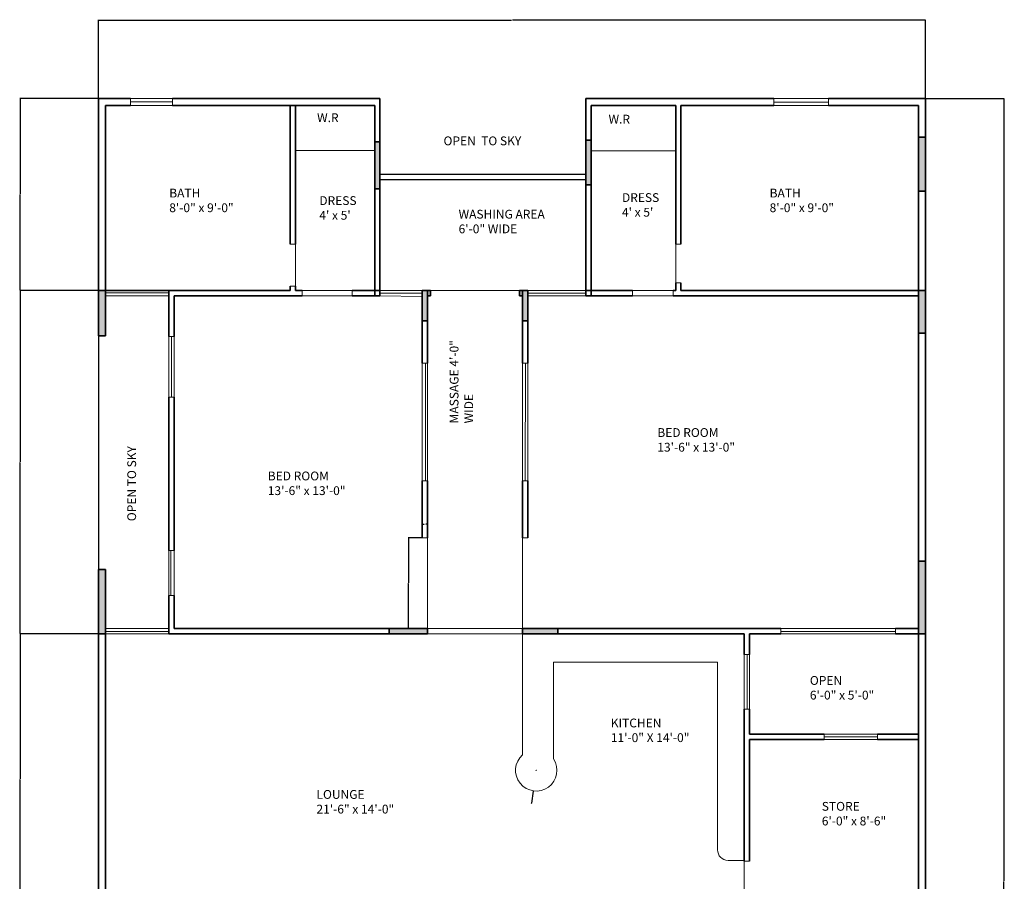
# Model space of a CAD drawing. Units: inches. Extents: x 1002 to 1561, y 1016 to 1994.
# Tile 8 of 8: x 1002 to 1561, y 1505 to 1994. Entities that reach past the tile are written whole.
import ezdxf

# ---------------------------------------------------------------- set-up
doc = ezdxf.new("R2010")
doc.units = ezdxf.units.IN
doc.header["$MEASUREMENT"] = 0
for name, color, linetype, lineweight in [('A-ANNO-DIMS', 2, 'Continuous', 18), ('A-AREA-IDEN', 7, 'Continuous', 18), ('A-WALL', 7, 'Continuous', 35), ('A-WALL-PATT', 7, 'Continuous', 13)]:
    doc.layers.add(name, color=color, linetype=linetype, lineweight=lineweight)
for name, color, linetype, lineweight, true_color in [('A-DOOR', 30, 'Continuous', 18, 0xf8991e), ('A-FLOR-CASE', 217, 'Continuous', 20, 0x93278f), ('A-FLOR-EDGE', 217, 'Continuous', 25, 0x93278f), ('A-GLAZ', 217, 'Continuous', 18, 0x93278f)]:
    doc.layers.add(name, color=color, linetype=linetype, lineweight=lineweight, true_color=true_color)
doc.styles.get("Standard").update_dxf_attribs({"font": 'arial.ttf'})
doc.dimstyles.get("Standard").update_dxf_attribs({"dimtxt": 0.18, "dimasz": 0.18, "dimexe": 0.18, "dimexo": 0.0625, "dimgap": 0.09, "dimtad": 0, "dimtih": 1, "dimtoh": 1, "dimdec": 4, "dimzin": 0, "dimdsep": 46, "dimtxsty": 'Standard', "dimcen": 0.09, "dimadec": 0, "dimazin": 0, "dimtfac": 1, "dimtdec": 4, "dimtofl": 0, "dimtmove": 0, "dimatfit": 3, "dimfxl": 1, "dimtolj": 1, "dimtzin": 0, "dimarcsym": 0})

# ---------------------------------------------------------------- blocks, each defined once
blk = doc.blocks.new('DOOR-PASSAGE-BEDROOM')
for p, q in [((0, 51.46), (3, 51.46)), ((3, 51.46), (3, 0))]:
    blk.add_line(p, q)
blk = doc.blocks.new('*D5')
at = {"layer": 'A-ANNO-DIMS', "color": 0, "lineweight": -2, "transparency": 16777216}
for p, q in [((1230.37, 1699.97), (1222.53, 1699.97)), ((1222.71, 1699.79), (1222.71, 1674.42)), ((1222.71, 1648.69), (1222.71, 1674.06)), ((1230.37, 1648.51), (1222.53, 1648.51))]:
    blk.add_line(p, q, dxfattribs=at)
at = {"layer": 'A-ANNO-DIMS', "color": 0, "transparency": 16777216}
for points in [[(1222.68, 1699.79), (1222.74, 1699.79), (1222.71, 1699.97)], [(1222.68, 1648.69), (1222.74, 1648.69), (1222.71, 1648.51)]]:
    blk.add_solid(points, dxfattribs=at)
at = {"layer": 'Defpoints', "color": 0, "transparency": 16777216}
for p in [(1222.71, 1699.97), (1230.43, 1699.97), (1230.43, 1648.51)]:
    blk.add_point(p, dxfattribs=at)
at = {"layer": 'A-ANNO-DIMS', "color": 0, "transparency": 16777216, "insert": (1222.71, 1674.24), "char_height": 0.18, "attachment_point": 5}
blk.add_mtext('\\A1;PASSAGE 51 TYP.', dxfattribs=at)
blk = doc.blocks.new('*D6')
at = {"layer": 'A-ANNO-DIMS', "color": 0, "lineweight": -2, "transparency": 16777216}
for p, q in [((1230.43, 1700.03), (1230.43, 1707.87)), ((1230.61, 1707.69), (1231.48, 1707.69)), ((1233.25, 1707.69), (1232.39, 1707.69)), ((1233.43, 1700.03), (1233.43, 1707.87))]:
    blk.add_line(p, q, dxfattribs=at)
at = {"layer": 'A-ANNO-DIMS', "color": 0, "transparency": 16777216}
for points in [[(1230.61, 1707.72), (1230.61, 1707.66), (1230.43, 1707.69)], [(1233.25, 1707.72), (1233.25, 1707.66), (1233.43, 1707.69)]]:
    blk.add_solid(points, dxfattribs=at)
at = {"layer": 'Defpoints', "color": 0, "transparency": 16777216}
for p in [(1233.43, 1707.69), (1230.43, 1699.97), (1233.43, 1699.97)]:
    blk.add_point(p, dxfattribs=at)
at = {"layer": 'A-ANNO-DIMS', "color": 0, "transparency": 16777216, "insert": (1231.93, 1707.69), "char_height": 0.18, "attachment_point": 5}
blk.add_mtext('\\A1;3 TYP.', dxfattribs=at)
blk = doc.blocks.new('*D7')
at = {"layer": 'A-ANNO-DIMS', "color": 0, "lineweight": -2, "transparency": 16777216}
for p, q in [((1046.43, 1949.57), (1046.43, 1994.2)), ((1046.61, 1994.02), (1281.14, 1994.02)), ((1516.25, 1994.02), (1281.73, 1994.02)), ((1516.43, 1949.57), (1516.43, 1994.2))]:
    blk.add_line(p, q, dxfattribs=at)
at = {"layer": 'A-ANNO-DIMS', "color": 0, "transparency": 16777216}
for points in [[(1046.61, 1994.05), (1046.61, 1993.99), (1046.43, 1994.02)], [(1516.25, 1994.05), (1516.25, 1993.99), (1516.43, 1994.02)]]:
    blk.add_solid(points, dxfattribs=at)
at = {"layer": 'Defpoints', "color": 0, "transparency": 16777216}
for p in [(1516.43, 1994.02), (1046.43, 1949.51), (1516.43, 1949.51)]:
    blk.add_point(p, dxfattribs=at)
at = {"layer": 'A-ANNO-DIMS', "color": 0, "transparency": 16777216, "insert": (1281.43, 1994.02), "char_height": 0.18, "attachment_point": 5}
blk.add_mtext('\\A1;470', dxfattribs=at)
blk = doc.blocks.new('*D8')
at = {"layer": 'A-ANNO-DIMS', "color": 0, "lineweight": -2, "transparency": 16777216}
for p, q in [((1516.5, 1949.51), (1561.12, 1949.51)), ((1560.94, 1949.33), (1560.94, 1505.18)), ((1560.94, 1060.67), (1560.94, 1504.82)), ((1472.5, 1060.49), (1561.12, 1060.49))]:
    blk.add_line(p, q, dxfattribs=at)
at = {"layer": 'A-ANNO-DIMS', "color": 0, "transparency": 16777216}
for points in [[(1560.91, 1949.33), (1560.97, 1949.33), (1560.94, 1949.51)], [(1560.91, 1060.67), (1560.97, 1060.67), (1560.94, 1060.49)]]:
    blk.add_solid(points, dxfattribs=at)
at = {"layer": 'Defpoints', "color": 0, "transparency": 16777216}
for p in [(1516.43, 1949.51), (1560.94, 1949.51), (1472.43, 1060.49)]:
    blk.add_point(p, dxfattribs=at)
at = {"layer": 'A-ANNO-DIMS', "color": 0, "transparency": 16777216, "insert": (1560.94, 1505), "char_height": 0.18, "attachment_point": 5}
blk.add_mtext('\\A1;889', dxfattribs=at)
blk = doc.blocks.new('*D9')
at = {"layer": 'A-ANNO-DIMS', "color": 0, "lineweight": -2, "transparency": 16777216}
for p, q in [((1046.37, 1949.51), (1001.74, 1949.51)), ((1001.92, 1949.33), (1001.92, 1895.19)), ((1001.92, 1840.69), (1001.92, 1894.83)), ((1046.37, 1840.51), (1001.74, 1840.51))]:
    blk.add_line(p, q, dxfattribs=at)
at = {"layer": 'A-ANNO-DIMS', "color": 0, "transparency": 16777216}
for points in [[(1001.89, 1949.33), (1001.95, 1949.33), (1001.92, 1949.51)], [(1001.89, 1840.69), (1001.95, 1840.69), (1001.92, 1840.51)]]:
    blk.add_solid(points, dxfattribs=at)
at = {"layer": 'Defpoints', "color": 0, "transparency": 16777216}
for p in [(1001.92, 1949.51), (1046.43, 1949.51), (1046.43, 1840.51)]:
    blk.add_point(p, dxfattribs=at)
at = {"layer": 'A-ANNO-DIMS', "color": 0, "transparency": 16777216, "insert": (1001.92, 1895.01), "char_height": 0.18, "attachment_point": 5}
blk.add_mtext('\\A1;109', dxfattribs=at)
blk = doc.blocks.new('*D10')
at = {"layer": 'A-ANNO-DIMS', "color": 0, "lineweight": -2, "transparency": 16777216}
for p, q in [((1046.37, 1840.51), (1001.74, 1840.51)), ((1001.92, 1840.33), (1001.92, 1743.19)), ((1001.92, 1645.69), (1001.92, 1742.83)), ((1046.37, 1645.51), (1001.74, 1645.51))]:
    blk.add_line(p, q, dxfattribs=at)
at = {"layer": 'A-ANNO-DIMS', "color": 0, "transparency": 16777216}
for points in [[(1001.89, 1840.33), (1001.95, 1840.33), (1001.92, 1840.51)], [(1001.89, 1645.69), (1001.95, 1645.69), (1001.92, 1645.51)]]:
    blk.add_solid(points, dxfattribs=at)
at = {"layer": 'Defpoints', "color": 0, "transparency": 16777216}
for p in [(1001.92, 1840.51), (1046.43, 1840.51), (1046.43, 1645.51)]:
    blk.add_point(p, dxfattribs=at)
at = {"layer": 'A-ANNO-DIMS', "color": 0, "transparency": 16777216, "insert": (1001.92, 1743.01), "char_height": 0.18, "attachment_point": 5}
blk.add_mtext('\\A1;195', dxfattribs=at)
blk = doc.blocks.new('*D11')
at = {"layer": 'A-ANNO-DIMS', "color": 0, "lineweight": -2, "transparency": 16777216}
for p, q in [((1046.37, 1645.51), (1001.74, 1645.51)), ((1001.92, 1645.33), (1001.92, 1563.19)), ((1001.92, 1480.69), (1001.92, 1562.83)), ((1046.37, 1480.51), (1001.74, 1480.51))]:
    blk.add_line(p, q, dxfattribs=at)
at = {"layer": 'A-ANNO-DIMS', "color": 0, "transparency": 16777216}
for points in [[(1001.89, 1645.33), (1001.95, 1645.33), (1001.92, 1645.51)], [(1001.89, 1480.69), (1001.95, 1480.69), (1001.92, 1480.51)]]:
    blk.add_solid(points, dxfattribs=at)
at = {"layer": 'Defpoints', "color": 0, "transparency": 16777216}
for p in [(1001.92, 1645.51), (1046.43, 1645.51), (1046.43, 1480.51)]:
    blk.add_point(p, dxfattribs=at)
at = {"layer": 'A-ANNO-DIMS', "color": 0, "transparency": 16777216, "insert": (1001.92, 1563.01), "char_height": 0.18, "attachment_point": 5}
blk.add_mtext('\\A1;165', dxfattribs=at)
blk = doc.blocks.new('*D22')
at = {"layer": 'A-ANNO-DIMS', "color": 0, "lineweight": -2, "transparency": 16777216}
for p, q in [((1295.12, 1568.03), (1295.3, 1568.03)), ((1295.21, 1567.94), (1295.21, 1568.12)), ((1292.67, 1549.35), (1293.6, 1556.18)), ((1292.49, 1549.35), (1292.67, 1549.35))]:
    blk.add_line(p, q, dxfattribs=at)
at = {"layer": 'A-ANNO-DIMS', "color": 0, "transparency": 16777216}
blk.add_solid([(1293.57, 1556.18), (1293.63, 1556.17), (1293.63, 1556.35)], dxfattribs=at)
at = {"layer": 'Defpoints', "color": 0, "transparency": 16777216}
for p in [(1295.21, 1568.03), (1293.63, 1556.35)]:
    blk.add_point(p, dxfattribs=at)
at = {"layer": 'A-ANNO-DIMS', "color": 0, "transparency": 16777216, "insert": (1292.01, 1549.35), "char_height": 0.18, "attachment_point": 5}
blk.add_mtext('\\A1;R11.78', dxfattribs=at)

msp = doc.modelspace()

# ---------------------------------------------------------------- hatches: boundary and pattern name
at = {"layer": 'A-WALL-PATT'}
h = msp.add_hatch(color=256, dxfattribs=at)
h.dxf.hatch_style = 1
h.paths.add_polyline_path([(1206.434, 1924.784), (1203.434, 1924.784), (1203.434, 1898.155), (1206.434, 1898.155)])
h.paths.add_polyline_path([(1326.434, 1925.745), (1323.434, 1925.745), (1323.434, 1900.458), (1326.434, 1900.458)])
h.paths.add_polyline_path([(1290.434, 1840.51), (1287.434, 1840.51), (1287.434, 1837.51), (1287.434, 1823.284), (1290.434, 1823.284)])
h.paths.add_polyline_path([(1287.434, 1840.51), (1285.684, 1840.51), (1285.684, 1837.51), (1287.434, 1837.51)])
h.paths.add_polyline_path([(1233.434, 1840.51), (1230.434, 1840.51), (1230.434, 1823.284), (1233.434, 1823.284)])
h.paths.add_polyline_path([(1235.119, 1840.51), (1233.434, 1840.51), (1233.434, 1837.51), (1235.119, 1837.51)])
h.paths.add_polyline_path([(1050.434, 1837.51), (1050.434, 1840.51), (1046.434, 1840.51), (1046.434, 1814.619), (1050.434, 1814.619)])
h.paths.add_polyline_path([(1050.434, 1682.088), (1046.434, 1682.088), (1046.434, 1648.51), (1046.434, 1645.51), (1050.434, 1645.51), (1050.434, 1648.51)])
h.paths.add_polyline_path([(1233.434, 1648.51), (1211.636, 1648.51), (1211.636, 1645.51), (1233.434, 1645.51)])
h.paths.add_polyline_path([(1307.549, 1648.51), (1287.434, 1648.51), (1287.434, 1645.51), (1307.549, 1645.51)])
h.paths.add_polyline_path([(1516.434, 1927.595), (1512.434, 1927.595), (1512.434, 1896.846), (1516.434, 1896.846)])
h.paths.add_polyline_path([(1516.434, 1840.51), (1512.434, 1840.51), (1512.434, 1816.31), (1516.434, 1816.31)])
h.paths.add_polyline_path([(1516.434, 1686.827), (1512.434, 1686.827), (1512.434, 1645.51), (1516.434, 1645.51)])
h.paths.add_polyline_path([(1472.434, 1321.51), (1469.434, 1321.51), (1469.434, 1306.51), (1472.434, 1306.51)])
h.paths.add_polyline_path([(1295.733, 1141.51), (1281.793, 1141.51), (1281.793, 1137.51), (1295.733, 1137.51)])
h.paths.add_polyline_path([(1239.434, 1321.51), (1230.434, 1321.51), (1230.434, 1318.51), (1239.434, 1318.51)])
h.paths.add_polyline_path([(1290.434, 1332.122), (1287.434, 1332.122), (1287.434, 1318.51), (1290.434, 1318.51)])
h.paths.add_polyline_path([(1311.434, 1480.51), (1287.434, 1480.51), (1287.434, 1477.51), (1311.434, 1477.51)])
h.paths.add_polyline_path([(1050.434, 1480.51), (1046.434, 1480.51), (1046.434, 1468.51), (1050.434, 1468.51)])
h.paths.add_polyline_path([(1050.434, 1321.51), (1046.434, 1321.51), (1046.434, 1309.51), (1050.434, 1309.51)])
h.paths.add_polyline_path([(1233.434, 1192.382), (1230.434, 1192.382), (1230.434, 1168.702), (1233.434, 1168.702)])
h.paths.add_polyline_path([(1050.434, 1137.51), (1046.434, 1137.51), (1046.434, 1119.51), (1050.434, 1119.51)])
h.paths.add_polyline_path([(1472.434, 1153.51), (1469.434, 1153.51), (1469.434, 1141.51), (1472.434, 1141.51)])
h.paths.add_polyline_path([(1472.434, 1141.51), (1469.434, 1141.51), (1469.434, 1137.51), (1472.434, 1137.51)])

# ---------------------------------------------------------------- linework, layer by layer
at = {"layer": 'A-DOOR'}
for p, q in [((1155.434, 1866.825), (1158.434, 1866.825)), ((1158.434, 1866.825), (1158.434, 1842.825)), ((1374.434, 1866.761), (1377.434, 1866.761)), ((1374.434, 1866.761), (1374.434, 1844.738)), ((1377.434, 1866.761), (1377.434, 1866.761)), ((1155.434, 1842.825), (1158.434, 1842.825)), ((1158.434, 1842.825), (1158.434, 1844.508)), ((1374.434, 1844.738), (1377.434, 1844.738)), ((1162.17, 1840.51), (1162.17, 1837.51)), ((1162.17, 1837.51), (1162.17, 1840.51)), ((1162.17, 1840.51), (1190.563, 1840.51)), ((1162.17, 1837.51), (1162.17, 1838.97)), ((1162.17, 1837.51), (1162.17, 1837.51)), ((1190.563, 1837.51), (1162.17, 1837.51)), ((1190.563, 1840.51), (1190.563, 1837.51)), ((1190.563, 1840.51), (1190.563, 1840.51)), ((1190.563, 1840.51), (1190.563, 1837.51)), ((1230.434, 1840.51), (1290.434, 1840.51)), ((1349.824, 1840.51), (1349.824, 1837.51)), ((1349.824, 1840.51), (1373.044, 1840.51)), ((1349.824, 1837.51), (1349.824, 1840.51)), ((1373.044, 1837.51), (1349.824, 1837.51)), ((1373.044, 1840.51), (1373.044, 1837.51)), ((1373.044, 1840.51), (1373.044, 1837.51)), ((1233.434, 1648.51), (1287.434, 1648.51)), ((1233.434, 1648.51), (1233.434, 1648.51)), ((1233.434, 1645.51), (1287.434, 1645.51)), ((1413.434, 1482.91), (1413.434, 1516.898)), ((1413.434, 1516.51), (1416.434, 1516.51))]:
    msp.add_line(p, q, dxfattribs=at)
at = {"layer": 'A-FLOR-CASE'}
for p, q in [((1158.434, 1919.94), (1203.434, 1919.94)), ((1326.434, 1919.822), (1374.434, 1919.822)), ((1287.434, 1645.51), (1287.434, 1576.873)), ((1305.105, 1574.472), (1305.105, 1629.469)), ((1305.105, 1629.469), (1398.202, 1629.469)), ((1398.202, 1629.469), (1398.202, 1522.898)), ((1305.075, 1574.472), (1305.105, 1574.472)), ((1404.202, 1516.898), (1413.434, 1516.898))]:
    msp.add_line(p, q, dxfattribs=at)
for centre, radius, start, end in [((1295.214, 1568.028), 11.78, 131.33697, 33.16787), ((1404.202, 1522.898), 6, 180, 270)]:
    msp.add_arc(centre, radius, start, end, dxfattribs=at)
at = {"layer": 'A-FLOR-EDGE'}
for p, q in [((1206.434, 1906.51), (1323.434, 1906.51)), ((1206.434, 1903.51), (1323.434, 1903.51)), ((1046.434, 1814.619), (1046.434, 1682.088))]:
    msp.add_line(p, q, dxfattribs=at)
at = {"layer": 'A-GLAZ'}
for p, q in [((1064.589, 1949.51), (1064.589, 1945.51)), ((1064.589, 1949.51), (1064.589, 1947.605)), ((1064.589, 1949.51), (1088.589, 1949.51)), ((1064.589, 1947.605), (1064.589, 1949.51)), ((1064.589, 1945.51), (1064.589, 1947.605)), ((1064.589, 1947.605), (1088.589, 1947.605)), ((1088.589, 1947.605), (1064.589, 1947.605)), ((1088.589, 1949.51), (1088.589, 1945.51)), ((1088.589, 1949.51), (1088.589, 1945.51)), ((1088.589, 1947.605), (1088.589, 1947.605)), ((1430.22, 1949.51), (1430.22, 1945.51)), ((1430.22, 1949.51), (1461.269, 1949.51)), ((1430.22, 1945.51), (1430.22, 1947.309)), ((1430.22, 1947.309), (1461.269, 1947.309)), ((1430.22, 1947.309), (1430.22, 1945.51)), ((1461.269, 1945.51), (1461.269, 1949.51)), ((1461.269, 1949.51), (1461.269, 1945.51)), ((1461.269, 1949.51), (1461.269, 1947.309)), ((1461.269, 1947.309), (1461.269, 1946.212)), ((1088.589, 1945.51), (1064.589, 1945.51)), ((1461.269, 1945.51), (1430.22, 1945.51)), ((1461.269, 1946.212), (1461.269, 1945.51)), ((1050.434, 1840.51), (1086.434, 1840.51)), ((1050.434, 1837.51), (1050.434, 1840.51)), ((1050.434, 1840.51), (1050.434, 1839.081)), ((1050.434, 1839.081), (1086.434, 1839.081)), ((1050.434, 1839.081), (1086.434, 1839.081)), ((1050.434, 1837.51), (1086.434, 1837.51)), ((1086.434, 1837.51), (1050.434, 1837.51)), ((1086.434, 1840.51), (1086.434, 1837.51)), ((1086.434, 1837.51), (1086.434, 1840.51)), ((1206.434, 1840.51), (1230.434, 1840.51)), ((1206.434, 1837.51), (1206.434, 1838.841)), ((1206.434, 1838.841), (1230.434, 1838.841)), ((1206.434, 1838.841), (1206.434, 1837.51)), ((1230.434, 1837.06), (1206.434, 1837.51)), ((1230.434, 1840.51), (1230.434, 1837.06)), ((1230.434, 1840.51), (1230.434, 1837.06)), ((1290.434, 1840.51), (1323.434, 1840.51)), ((1290.434, 1837.51), (1290.434, 1838.931)), ((1290.434, 1838.931), (1323.434, 1838.931)), ((1290.434, 1838.931), (1290.434, 1837.51)), ((1323.434, 1837.51), (1290.434, 1837.51)), ((1323.434, 1840.51), (1323.434, 1837.51)), ((1086.434, 1814.37), (1089.434, 1814.37)), ((1086.434, 1814.37), (1086.434, 1779.843)), ((1089.434, 1814.37), (1087.973, 1814.37)), ((1087.973, 1814.37), (1087.973, 1779.843)), ((1089.434, 1779.843), (1089.434, 1814.37)), ((1230.434, 1799.12), (1233.434, 1799.12)), ((1230.434, 1799.12), (1230.434, 1732.434)), ((1233.434, 1799.12), (1232.301, 1799.12)), ((1233.434, 1799.12), (1232.301, 1799.12)), ((1232.301, 1799.12), (1232.301, 1732.434)), ((1233.434, 1799.12), (1232.301, 1799.12)), ((1233.434, 1732.434), (1233.434, 1799.12)), ((1287.434, 1799.12), (1290.434, 1799.12)), ((1287.434, 1799.12), (1290.434, 1799.12)), ((1287.434, 1732.434), (1287.434, 1799.12)), ((1287.434, 1799.12), (1290.434, 1799.12)), ((1288.984, 1732.434), (1289.17, 1799.12)), ((1290.434, 1799.12), (1289.17, 1799.12)), ((1290.434, 1799.12), (1290.434, 1732.434)), ((1086.434, 1779.843), (1089.434, 1779.843)), ((1086.434, 1779.843), (1089.434, 1779.843)), ((1230.434, 1732.434), (1233.434, 1732.434)), ((1230.434, 1732.434), (1233.434, 1732.434)), ((1230.434, 1732.434), (1233.434, 1732.434)), ((1287.434, 1732.434), (1290.434, 1732.434)), ((1290.434, 1732.434), (1287.434, 1732.434)), ((1287.434, 1732.434), (1288.984, 1732.434)), ((1288.984, 1732.434), (1287.434, 1732.434)), ((1287.434, 1732.434), (1288.984, 1732.434)), ((1287.434, 1732.434), (1288.984, 1732.434)), ((1288.984, 1732.434), (1287.434, 1732.434)), ((1287.434, 1732.434), (1288.984, 1732.434)), ((1288.984, 1732.434), (1287.434, 1732.434)), ((1287.434, 1732.434), (1287.434, 1732.434)), ((1287.434, 1732.434), (1290.434, 1732.434)), ((1290.434, 1732.434), (1288.984, 1732.434)), ((1089.434, 1692.845), (1086.434, 1692.845)), ((1086.434, 1692.845), (1086.434, 1667.256)), ((1089.434, 1692.845), (1087.651, 1692.845)), ((1087.651, 1692.845), (1087.651, 1667.256)), ((1089.434, 1667.256), (1089.434, 1692.845)), ((1086.434, 1667.256), (1089.434, 1667.256)), ((1086.434, 1667.256), (1089.434, 1667.256)), ((1050.434, 1648.51), (1050.434, 1648.51)), ((1086.434, 1648.51), (1050.434, 1648.51)), ((1050.434, 1648.51), (1050.434, 1645.51)), ((1050.434, 1645.51), (1050.434, 1646.847)), ((1050.434, 1646.847), (1086.434, 1646.847)), ((1050.434, 1645.51), (1086.434, 1645.51)), ((1086.434, 1645.51), (1086.434, 1648.51)), ((1086.434, 1648.51), (1086.434, 1645.51)), ((1086.434, 1648.51), (1086.434, 1645.51)), ((1086.434, 1648.51), (1086.434, 1645.51)), ((1434.192, 1648.51), (1434.192, 1645.51)), ((1434.192, 1648.51), (1499.306, 1648.51)), ((1434.192, 1645.51), (1434.192, 1646.91)), ((1434.192, 1646.91), (1499.306, 1646.91)), ((1499.306, 1645.51), (1434.192, 1645.51)), ((1499.306, 1648.51), (1499.306, 1645.51)), ((1499.306, 1648.51), (1499.306, 1645.51)), ((1413.434, 1633.854), (1416.434, 1633.854)), ((1413.434, 1633.854), (1413.434, 1602.679)), ((1416.434, 1633.854), (1415.045, 1633.854)), ((1415.045, 1633.854), (1415.045, 1602.679)), ((1416.434, 1602.679), (1416.434, 1633.854)), ((1416.434, 1602.679), (1413.434, 1602.679)), ((1413.434, 1602.679), (1416.434, 1602.679)), ((1458.847, 1588.51), (1458.847, 1585.51)), ((1458.847, 1588.51), (1489.017, 1588.51)), ((1458.847, 1586.362), (1458.847, 1587.066)), ((1458.847, 1587.066), (1489.017, 1587.066)), ((1458.847, 1585.51), (1458.847, 1586.362)), ((1489.017, 1585.51), (1458.847, 1585.51)), ((1489.017, 1585.51), (1489.017, 1588.51)), ((1489.017, 1588.51), (1489.017, 1585.51))]:
    msp.add_line(p, q, dxfattribs=at)
at = {"layer": 'A-WALL'}
for p, q in [((1046.434, 1949.51), (1064.589, 1949.51)), ((1046.434, 1949.51), (1064.589, 1949.51)), ((1046.434, 1949.51), (1046.434, 1814.619)), ((1046.434, 1814.619), (1046.434, 1949.51)), ((1088.589, 1949.51), (1206.434, 1949.51)), ((1206.434, 1837.51), (1206.434, 1949.51)), ((1323.434, 1837.51), (1323.434, 1949.51)), ((1323.434, 1949.51), (1430.22, 1949.51)), ((1323.434, 1949.51), (1323.434, 1925.745)), ((1516.434, 1949.51), (1461.269, 1949.51)), ((1461.269, 1949.51), (1516.434, 1949.51)), ((1516.434, 1949.51), (1516.434, 1927.595)), ((1050.434, 1945.51), (1064.589, 1945.51)), ((1050.434, 1945.51), (1050.434, 1839.081)), ((1088.589, 1945.51), (1203.434, 1945.51)), ((1155.434, 1866.825), (1155.434, 1945.51)), ((1158.434, 1945.51), (1158.434, 1927.313)), ((1158.434, 1945.51), (1158.434, 1909.558)), ((1158.434, 1866.825), (1158.434, 1945.51)), ((1203.434, 1837.51), (1203.434, 1945.51)), ((1203.434, 1945.51), (1203.434, 1898.155)), ((1326.434, 1837.51), (1326.434, 1945.51)), ((1326.434, 1945.51), (1374.434, 1945.51)), ((1326.434, 1945.51), (1326.434, 1919.822)), ((1374.434, 1866.761), (1374.434, 1945.51)), ((1377.434, 1866.761), (1377.434, 1945.51)), ((1377.434, 1945.51), (1430.22, 1945.51)), ((1461.269, 1945.51), (1512.434, 1945.51)), ((1512.434, 1945.51), (1512.434, 1480.51)), ((1512.434, 1945.51), (1512.434, 1927.595)), ((1203.434, 1927.313), (1203.434, 1927.313)), ((1206.434, 1924.784), (1203.434, 1924.784)), ((1206.434, 1898.155), (1206.434, 1924.784)), ((1206.434, 1924.784), (1206.434, 1924.784)), ((1323.434, 1925.745), (1326.434, 1925.745)), ((1323.434, 1900.458), (1323.434, 1925.745)), ((1326.434, 1925.745), (1326.434, 1900.458)), ((1512.434, 1927.595), (1516.434, 1927.595)), ((1512.434, 1896.846), (1512.434, 1927.595)), ((1516.434, 1927.595), (1516.434, 1896.846)), ((1158.434, 1909.558), (1158.434, 1919.94)), ((1374.434, 1919.822), (1374.434, 1919.822)), ((1203.434, 1898.155), (1206.434, 1898.155)), ((1206.434, 1898.155), (1206.434, 1898.155)), ((1326.434, 1900.458), (1323.434, 1900.458)), ((1326.434, 1900.458), (1326.434, 1900.458)), ((1516.434, 1896.846), (1512.434, 1896.846)), ((1516.434, 1896.846), (1516.434, 1840.51)), ((1155.434, 1840.51), (1155.434, 1842.825)), ((1155.434, 1840.51), (1155.434, 1842.825)), ((1158.434, 1840.51), (1158.434, 1842.825)), ((1374.434, 1840.51), (1374.434, 1844.738)), ((1374.434, 1840.51), (1374.434, 1844.738)), ((1374.434, 1840.51), (1374.434, 1844.738)), ((1377.434, 1840.51), (1377.434, 1844.738)), ((1050.434, 1840.51), (1046.434, 1840.51)), ((1050.434, 1840.51), (1155.434, 1840.51)), ((1050.434, 1837.51), (1050.434, 1840.51)), ((1050.434, 1837.51), (1050.434, 1814.619)), ((1086.434, 1840.51), (1086.434, 1814.37)), ((1086.434, 1840.51), (1086.434, 1814.37)), ((1086.434, 1814.37), (1086.434, 1840.51)), ((1089.434, 1837.51), (1162.17, 1837.51)), ((1089.434, 1814.37), (1089.434, 1837.51)), ((1158.434, 1840.51), (1162.17, 1840.51)), ((1158.434, 1840.51), (1162.17, 1840.51)), ((1162.17, 1840.51), (1158.434, 1840.51)), ((1158.434, 1840.51), (1162.17, 1840.51)), ((1190.563, 1840.51), (1206.434, 1840.51)), ((1190.563, 1837.51), (1206.434, 1837.51)), ((1230.434, 1840.51), (1235.119, 1840.51)), ((1230.434, 1840.51), (1233.434, 1840.51)), ((1230.434, 1840.51), (1230.434, 1823.284)), ((1230.434, 1840.51), (1230.434, 1799.12)), ((1230.434, 1799.12), (1230.434, 1840.51)), ((1233.434, 1799.12), (1233.434, 1840.51)), ((1233.434, 1837.51), (1235.119, 1837.51)), ((1235.119, 1840.51), (1235.119, 1837.51)), ((1290.434, 1840.51), (1285.684, 1840.51)), ((1285.684, 1840.51), (1285.684, 1837.51)), ((1285.684, 1837.51), (1287.434, 1837.51)), ((1287.434, 1837.51), (1287.434, 1840.51)), ((1287.434, 1799.12), (1287.434, 1840.51)), ((1290.434, 1799.12), (1290.434, 1840.51)), ((1323.434, 1840.51), (1349.824, 1840.51)), ((1323.434, 1837.51), (1349.824, 1837.51)), ((1374.434, 1840.51), (1373.044, 1840.51)), ((1374.434, 1840.51), (1373.044, 1840.51)), ((1373.044, 1840.51), (1374.434, 1840.51)), ((1373.044, 1837.51), (1512.434, 1837.51)), ((1377.434, 1840.51), (1512.434, 1840.51)), ((1512.434, 1840.51), (1516.434, 1840.51)), ((1512.434, 1816.31), (1512.434, 1840.51)), ((1516.434, 1840.51), (1516.434, 1816.31)), ((1230.434, 1823.284), (1233.434, 1823.284)), ((1287.434, 1823.284), (1290.434, 1823.284)), ((1046.434, 1814.619), (1046.434, 1814.619)), ((1046.434, 1814.619), (1046.434, 1814.619)), ((1046.434, 1814.619), (1050.434, 1814.619)), ((1516.434, 1816.31), (1512.434, 1816.31)), ((1516.434, 1816.31), (1516.434, 1686.827)), ((1086.434, 1692.845), (1086.434, 1779.843)), ((1089.434, 1692.845), (1089.434, 1779.843)), ((1230.434, 1732.434), (1230.434, 1699.969)), ((1230.434, 1699.969), (1230.434, 1732.434)), ((1230.434, 1699.969), (1230.434, 1732.434)), ((1233.434, 1699.969), (1233.434, 1732.434)), ((1287.434, 1699.969), (1287.434, 1732.434)), ((1290.434, 1699.969), (1290.434, 1732.434)), ((1516.434, 1686.827), (1512.434, 1686.827)), ((1512.434, 1686.827), (1512.434, 1645.51)), ((1516.434, 1645.51), (1516.434, 1686.827)), ((1046.434, 1119.51), (1046.434, 1682.088)), ((1046.434, 1648.51), (1046.434, 1682.088)), ((1046.434, 1682.088), (1050.434, 1682.088)), ((1050.434, 1119.51), (1050.434, 1682.088)), ((1050.434, 1682.088), (1050.434, 1645.51)), ((1086.434, 1665.82), (1086.434, 1667.256)), ((1089.434, 1667.256), (1089.434, 1666.685)), ((1086.434, 1645.51), (1086.434, 1666.685)), ((1086.434, 1645.51), (1086.434, 1666.685)), ((1086.434, 1645.51), (1086.434, 1665.82)), ((1089.434, 1648.51), (1089.434, 1666.685)), ((1046.434, 1648.51), (1046.434, 1652.338)), ((1046.434, 1645.51), (1046.434, 1648.51)), ((1050.434, 1645.51), (1046.434, 1645.51)), ((1050.434, 1648.51), (1050.434, 1645.51)), ((1086.434, 1645.51), (1233.434, 1645.51)), ((1089.434, 1648.51), (1233.434, 1648.51)), ((1233.434, 1648.51), (1211.636, 1648.51)), ((1211.636, 1648.51), (1211.636, 1645.51)), ((1233.434, 1648.51), (1211.636, 1648.51)), ((1211.636, 1645.51), (1233.434, 1645.51)), ((1233.434, 1645.51), (1233.434, 1648.51)), ((1233.434, 1645.51), (1233.434, 1648.51)), ((1287.434, 1645.51), (1287.434, 1648.51)), ((1287.434, 1645.51), (1287.434, 1648.51)), ((1287.434, 1648.51), (1434.192, 1648.51)), ((1287.434, 1648.51), (1307.549, 1648.51)), ((1287.434, 1645.51), (1287.434, 1648.51)), ((1287.434, 1645.51), (1413.434, 1645.51)), ((1307.549, 1645.51), (1287.434, 1645.51)), ((1307.549, 1648.51), (1307.549, 1645.51)), ((1413.434, 1645.51), (1413.434, 1633.854)), ((1413.434, 1645.51), (1413.434, 1633.854)), ((1413.434, 1633.854), (1413.434, 1645.51)), ((1416.434, 1645.51), (1416.434, 1633.854)), ((1416.434, 1645.51), (1434.192, 1645.51)), ((1416.434, 1633.854), (1416.434, 1645.51)), ((1512.434, 1648.51), (1499.306, 1648.51)), ((1512.434, 1648.51), (1499.306, 1648.51)), ((1499.306, 1648.51), (1512.434, 1648.51)), ((1499.306, 1645.51), (1512.434, 1645.51)), ((1512.434, 1645.51), (1516.434, 1645.51)), ((1516.434, 1645.51), (1516.434, 1387.504)), ((1413.434, 1602.679), (1413.434, 1516.51)), ((1413.434, 1516.51), (1413.434, 1602.679)), ((1416.434, 1602.679), (1416.434, 1588.51)), ((1416.434, 1588.51), (1416.434, 1602.679)), ((1416.434, 1588.51), (1458.847, 1588.51)), ((1416.434, 1588.51), (1458.847, 1588.51)), ((1416.434, 1585.51), (1458.847, 1585.51)), ((1416.434, 1585.51), (1416.434, 1516.51)), ((1416.434, 1516.51), (1416.434, 1585.51)), ((1489.017, 1588.51), (1512.434, 1588.51)), ((1489.017, 1585.51), (1512.434, 1585.51))]:
    msp.add_line(p, q, dxfattribs=at)
msp.add_lwpolyline([(1086.434, 1837.51), (1086.293, 1837.51)], dxfattribs=at)

# ---------------------------------------------------------------- block references
at = {"layer": 'A-DOOR'}
msp.add_blockref('DOOR-PASSAGE-BEDROOM', (1230.434, 1648.51), dxfattribs=at)
at = {"layer": 'A-DOOR', "extrusion": (0, 0, -1), "zscale": -1}
msp.add_blockref('DOOR-PASSAGE-BEDROOM', (-1290.433, 1648.51), dxfattribs=at)

# ---------------------------------------------------------------- texts
at = {"layer": 'A-AREA-IDEN', "char_height": 5, "attachment_point": 1}
for s, width, insert in [('W.R', 50.5101, (1170.686, 1941.055)), ('W.R', 50.5101, (1336.292, 1940.229)), ('OPEN  TO SKY', 50.5101, (1242.52, 1927.908)), ('BATH\\P8\'-0" x 9\'-0"', 50.5101, (1086.692, 1898.263)), ('BATH\\P8\'-0" x 9\'-0"', 50.5101, (1427.804, 1898.263)), ("DRESS\\P4' x 5'", 50.5101, (1171.959, 1893.985)), ("DRESS\\P4' x 5'", 50.5101, (1343.914, 1895.706)), ('WASHING AREA\\P6\'-0" WIDE', 58.97229, (1251.092, 1886.273)), ('BED ROOM\\P13\'-6" x 13\'-0"', 50.5101, (1364.008, 1762.297)), ('BED ROOM\\P13\'-6" x 13\'-0"', 50.5101, (1142.674, 1737.638)), ('OPEN\\P6\'-0" x 5\'-0"', 50.5101, (1450.673, 1621.534)), ('KITCHEN\\P11\'-0" X 14\'-0"', 50.5101, (1337.574, 1597.387)), ('LOUNGE\\P21\'-6" x 14\'-0"', 50.5101, (1170.343, 1556.821)), ('STORE\\P6\'-0" x 8\'-6"', 50.5101, (1457.439, 1550.06))]:
    msp.add_mtext_dynamic_manual_height_columns(s, width=width, gutter_width=1, heights=[0], dxfattribs=dict(at, insert=insert))
at = {"layer": 'A-AREA-IDEN', "char_height": 5, "attachment_point": 1, "rotation": 90}
for s, insert in [('MASSAGE 4\'-0" WIDE', (1246.033, 1764.994)), ('OPEN TO SKY', (1062.855, 1709.454))]:
    msp.add_mtext_dynamic_manual_height_columns(s, width=50.5101, gutter_width=1, heights=[0], dxfattribs=dict(at, insert=insert))

# ---------------------------------------------------------------- dimensions: what is measured, and where the dimension line sits
at = {"layer": 'A-ANNO-DIMS'}
dim = msp.add_linear_dim(base=(1516.434, 1994.02), p1=(1046.434, 1949.51), p2=(1516.434, 1949.51), dimstyle='Standard', override={"dimdec": 0, "dimlfac": 1, "dimrnd": 0, "dimzin": 0, "dimdsep": 46, "dimlunit": 2}, dxfattribs=at)
dim.commit()
dim.dimension.update_dxf_attribs({"geometry": '*D7', "text_midpoint": (1281.434, 1994.02)})
for base, p1, p2, picture, middle in [((1001.924, 1949.51), (1046.434, 1840.51), (1046.434, 1949.51), '*D9', (1001.924, 1895.01)), ((1560.944, 1949.51), (1472.434, 1060.49), (1516.434, 1949.51), '*D8', (1560.944, 1505)), ((1001.924, 1840.51), (1046.434, 1645.51), (1046.434, 1840.51), '*D10', (1001.924, 1743.01)), ((1001.924, 1645.51), (1046.434, 1480.51), (1046.434, 1645.51), '*D11', (1001.924, 1563.01))]:
    dim = msp.add_linear_dim(base=base, p1=p1, p2=p2, angle=90, dimstyle='Standard', override={"dimdec": 0, "dimlfac": 1, "dimrnd": 0, "dimzin": 0, "dimdsep": 46, "dimlunit": 2}, dxfattribs=at)
    dim.commit()
    dim.dimension.update_dxf_attribs({"geometry": picture, "text_midpoint": middle})
dim = msp.add_linear_dim(base=(1233.434, 1707.688), p1=(1230.434, 1699.969), p2=(1233.434, 1699.969), text='<> TYP.', dimstyle='Standard', override={"dimdec": 0, "dimlfac": 1, "dimrnd": 0, "dimzin": 0, "dimdsep": 46, "dimlunit": 2}, dxfattribs=at)
dim.commit()
dim.dimension.update_dxf_attribs({"geometry": '*D6', "text_midpoint": (1231.934, 1707.688)})
dim = msp.add_linear_dim(base=(1222.715, 1699.969), p1=(1230.434, 1648.51), p2=(1230.434, 1699.969), angle=90, text='PASSAGE <> TYP.', dimstyle='Standard', override={"dimdec": 0, "dimlfac": 1, "dimrnd": 0, "dimzin": 0, "dimdsep": 46, "dimlunit": 2}, dxfattribs=at)
dim.commit()
dim.dimension.update_dxf_attribs({"geometry": '*D5', "text_midpoint": (1222.715, 1674.239)})
dim = msp.add_radius_dim(center=(1295.214, 1568.028), mpoint=(1293.626, 1556.355), dimstyle='Standard', override={"dimdec": 2, "dimlfac": 1, "dimrnd": 0, "dimzin": 0, "dimdsep": 46, "dimlunit": 2}, dxfattribs=at)
dim.commit()
dim.dimension.update_dxf_attribs({"geometry": '*D22', "text_midpoint": (1292.013, 1549.351), "dimtype": 164})

doc.saveas('drawing.dxf')
